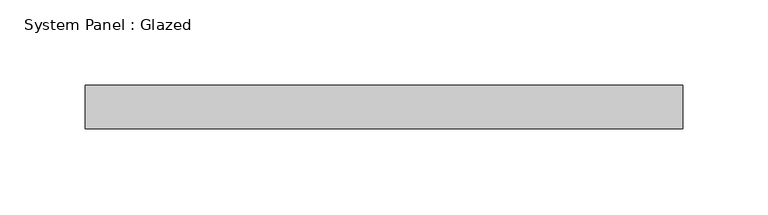
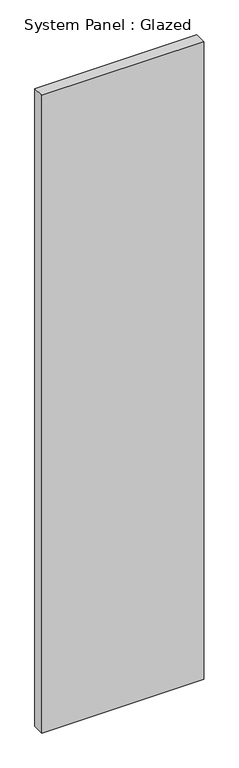
"""IFC4 building model written with IfcOpenShell, lengths in millimetres: plate geometry, System Panel : Glazed."""

from ifc_helpers import new_model, si_unit, origin, origin_with_axes, place, context, project, spatial, polyline, outline, extrude, source, transform, mapped, element, save


def system_panel_glazed_d6ecc329(model_context):
    return source(origin(), model_context, "Body", "SweptSolid", [
        extrude(outline(polyline([(174.625, 19.05), (-174.625, 19.05), (-174.625, 44.45), (174.625, 44.45), (174.625, 19.05)])), origin_with_axes(), (0.0, 0.0, 1.0), 1453.0534505),
    ])


if __name__ == "__main__":
    model = new_model("IFC4")
    model_context = context("Model", 3, world=origin())
    ifc_project = project(units=[si_unit("LENGTHUNIT", "METRE", prefix="MILLI")], contexts=[model_context])
    site = spatial("IfcSite", under=ifc_project)
    building = spatial("IfcBuilding", under=site)
    placement = place(None, origin())
    system_panel_glazed_shape = system_panel_glazed_d6ecc329(model_context)
    element("IfcPlate", 1, ObjectType="System Panel : Glazed", at=placement, inside=building, context=model_context, shape_type="MappedRepresentation", body=[
        mapped(system_panel_glazed_shape, transform((0.0, 0.0, 0.0), x_axis=(1.0, 0.0, 0.0), y_axis=(0.0, 1.0, 0.0), z_axis=(0.0, 0.0, 1.0))),
    ])
    save(model, "model.ifc")

# Revit data of these elements
# Type "System Panel : Glazed"
#   Construction Type Id = "GSP4R"
#   Analytic Construction = "1/8 in Pilkington single glazing"
#   Visual Light Transmittance = 0.9
#   Solar Heat Gain Coefficient = 0.86
#   Heat Transfer Coefficient (U) = 1.18115 BTU/(h·ft²·°F)
#   Define Thermal Properties by = 1
# Element 1 (IfcPlate, "System Panel : Glazed")
#   Materials on its faces: "Glass"
# Materials
#   "Glass": class "Glass", colour RGB 0 128 192, transparency 0.75, Description = "Soda Lime Glass", Cost = 0
